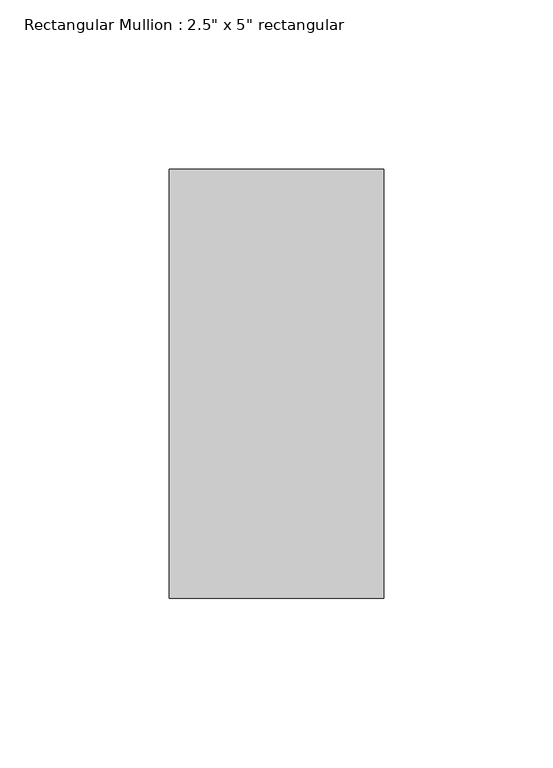
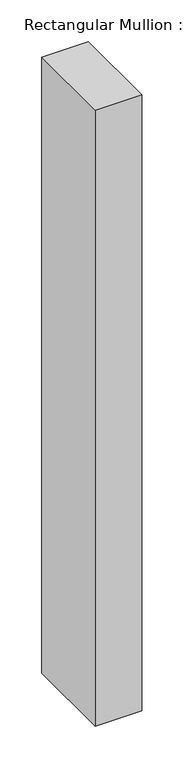
"""IFC4 building model written with IfcOpenShell, lengths in millimetres: member geometry."""

from ifc_helpers import new_model, si_unit, frame, origin, place, context, project, spatial, polyline, outline, extrude, source, transform, mapped, element, save


def member_e2125230(model_context):
    return source(origin(), model_context, "Body", "SweptSolid", [
        extrude(outline(polyline([(0.0, 63.5), (0.0, -63.5), (-63.5, -63.5), (-63.5, 63.5), (0.0, 63.5)])), frame((0.0, 0.0, -894.9490947), z_axis=(0.0, 0.0, 1.0), x_axis=(1.0, 0.0, 0.0)), (0.0, 0.0, 1.0), 894.9490947),
    ])


if __name__ == "__main__":
    model = new_model("IFC4")
    model_context = context("Model", 3, world=origin())
    ifc_project = project(units=[si_unit("LENGTHUNIT", "METRE", prefix="MILLI")], contexts=[model_context])
    site = spatial("IfcSite", under=ifc_project)
    building = spatial("IfcBuilding", under=site)
    placement = place(None, origin())
    member_shape = member_e2125230(model_context)
    element("IfcMember", 1, ObjectType="Rectangular Mullion : 2.5\" x 5\" rectangular", at=placement, inside=building, context=model_context, shape_type="MappedRepresentation", body=[
        mapped(member_shape, transform((0.0, 0.0, 0.0), x_axis=(1.0, 0.0, 0.0), y_axis=(0.0, 1.0, 0.0), z_axis=(0.0, 0.0, 1.0))),
    ])
    save(model, "model.ifc")

# Revit data of these elements
# Type "Rectangular Mullion : 2.5\" x 5\" rectangular"
#   built-in parameter 1007304 = 0.416667 (stored number, unit not read)
#   built-in parameter 1007301 = 0.104167 (stored number, unit not read)
#   built-in parameter 1007300 = 0.104167 (stored number, unit not read)
# Element 1 (IfcMember, "Rectangular Mullion : 2.5\" x 5\" rectangular")
#   Materials on its faces: "Aluminum"
# Materials
#   "Aluminum": class "Metal", colour RGB 247 247 247, transparency 0, Description = "Aluminum 6061", Cost = 0
